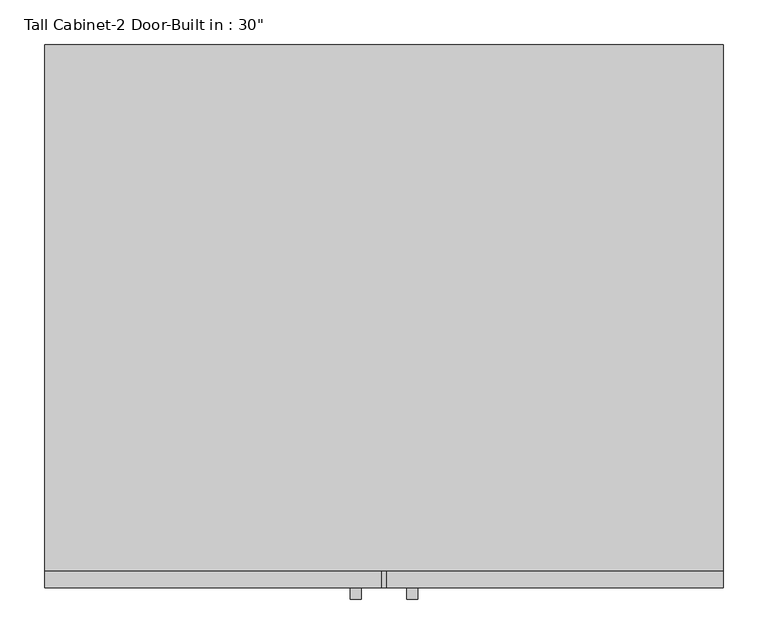
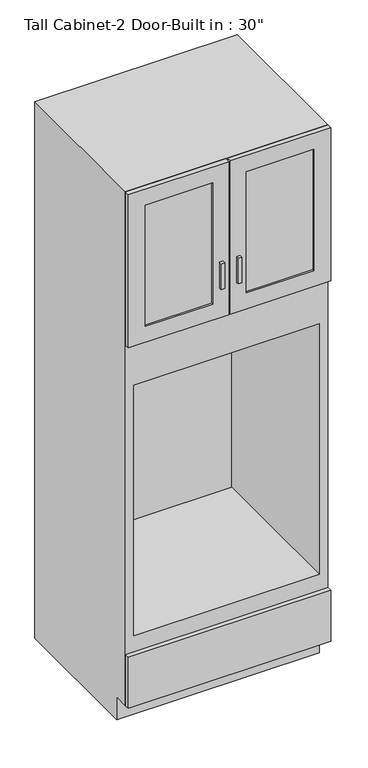
"""IFC4 building model written with IfcOpenShell, lengths in millimetres: furniture geometry."""

from ifc_helpers import new_model, si_unit, frame, origin, place, context, project, spatial, polyline, outline, extrude, faceted_brep, source, transform, mapped, element, save


def furniture_fb6977ac(model_context):
    return source(origin(), model_context, "Body", "SolidModel", [
        faceted_brep([(399.7377049, -590.55, 90.4875), (399.7377049, -590.55, 2135.1875), (-362.2622951, -590.55, 2135.1875), (-362.2622951, -590.55, 90.4875), (-343.2122951, -590.55, 2116.1375), (380.6877049, -590.55, 2116.1375), (380.6877049, -590.55, 1525.5875), (-343.2122951, -590.55, 1525.5875), (367.9877049, -590.55, 357.1875), (-330.5122951, -590.55, 357.1875), (-330.5122951, -590.55, 1354.1375), (367.9877049, -590.55, 1354.1375), (-362.2622951, 0.0, 2135.1875), (399.7377049, 0.0, 2135.1875), (399.7377049, 0.0, 0.0), (-362.2622951, 0.0, 0.0), (399.7377049, -533.4, 90.4875), (399.7377049, -533.4, 0.0), (-362.2622951, -533.4, 0.0), (-362.2622951, -533.4, 90.4875), (380.6877049, -19.05, 2116.1375), (380.6877049, -19.05, 1525.5875), (-343.2122951, -19.05, 1525.5875), (-343.2122951, -19.05, 2116.1375), (367.9877049, -19.05, 357.1875), (-330.5122951, -19.05, 357.1875), (-330.5122951, -19.05, 1354.1375), (367.9877049, -19.05, 1354.1375)], [[[0, 1, 2, 3], [4, 5, 6, 7], [8, 9, 10, 11]], [[12, 13, 14, 15]], [[1, 0, 16, 17, 14, 13]], [[2, 1, 13, 12]], [[3, 2, 12, 15, 18, 19]], [[0, 3, 19, 16]], [[6, 5, 20, 21]], [[4, 7, 22, 23]], [[5, 4, 23, 20]], [[14, 17, 18, 15]], [[18, 17, 16, 19]], [[7, 6, 21, 22]], [[9, 8, 24, 25]], [[10, 9, 25, 26]], [[11, 10, 26, 27]], [[8, 11, 27, 24]], [[21, 20, 23, 22]], [[25, 24, 27, 26]]]),
        extrude(outline(polyline([(399.7377049, -609.6), (-362.2622951, -609.6), (-362.2622951, -590.55), (399.7377049, -590.55), (399.7377049, -609.6)])), frame((0.0, 0.0, 90.4875), z_axis=(0.0, 0.0, 1.0), x_axis=(1.0, 0.0, 0.0)), (0.0, 0.0, 1.0), 203.2),
        extrude(outline(polyline([(2135.1875, 15.5627049), (2135.1875, -362.2622951), (1525.5875, -362.2622951), (1525.5875, 15.5627049), (2135.1875, 15.5627049)]), holes=[polyline([(2071.6875, -44.7622951), (1589.0875, -44.7622951), (1589.0875, -298.7622951), (2071.6875, -298.7622951), (2071.6875, -44.7622951)])]), frame((0.0, -609.6, 0.0), z_axis=(0.0, 1.0, 0.0), x_axis=(0.0, 0.0, 1.0)), (0.0, 0.0, 1.0), 19.05),
        extrude(outline(polyline([(2135.1875, 21.9127049), (1525.5875, 21.9127049), (1525.5875, 399.7377049), (2135.1875, 399.7377049), (2135.1875, 21.9127049)]), holes=[polyline([(2071.6875, 336.2377049), (1589.0875, 336.2377049), (1589.0875, 82.2377049), (2071.6875, 82.2377049), (2071.6875, 336.2377049)])]), frame((0.0, -609.6, 0.0), z_axis=(0.0, 1.0, 0.0), x_axis=(0.0, 0.0, 1.0)), (0.0, 0.0, 1.0), 19.05),
        extrude(outline(polyline([(399.7377049, -609.6), (-362.2622951, -609.6), (-362.2622951, -590.55), (399.7377049, -590.55), (399.7377049, -609.6)])), frame((0.0, 0.0, 90.4875), z_axis=(0.0, 0.0, 1.0), x_axis=(1.0, 0.0, 0.0)), (0.0, 0.0, 1.0), 203.2),
        extrude(outline(polyline([(-6.6622951, -622.3), (-19.1945267, -622.3), (-19.1945267, -609.6), (-6.6622951, -609.6), (-6.6622951, -622.3)])), frame((0.0, 0.0, 1645.6417867), z_axis=(0.0, 0.0, 1.0), x_axis=(1.0, 0.0, 0.0)), (0.0, 0.0, 1.0), 101.6),
        extrude(outline(polyline([(56.6699365, -622.3), (44.1377049, -622.3), (44.1377049, -609.6), (56.6699365, -609.6), (56.6699365, -622.3)])), frame((0.0, 0.0, 1645.6417867), z_axis=(0.0, 0.0, 1.0), x_axis=(1.0, 0.0, 0.0)), (0.0, 0.0, 1.0), 101.6),
        extrude(outline(polyline([(-44.7622951, -603.25), (-298.7622951, -603.25), (-298.7622951, -596.9), (-44.7622951, -596.9), (-44.7622951, -603.25)])), frame((0.0, 0.0, 1589.0875), z_axis=(0.0, 0.0, 1.0), x_axis=(1.0, 0.0, 0.0)), (0.0, 0.0, 1.0), 482.6),
        extrude(outline(polyline([(336.2377049, -603.25), (82.2377049, -603.25), (82.2377049, -596.9), (336.2377049, -596.9), (336.2377049, -603.25)])), frame((0.0, 0.0, 1589.0875), z_axis=(0.0, 0.0, 1.0), x_axis=(1.0, 0.0, 0.0)), (0.0, 0.0, 1.0), 482.6),
    ])


if __name__ == "__main__":
    model = new_model("IFC4")
    model_context = context("Model", 3, world=origin())
    ifc_project = project(units=[si_unit("LENGTHUNIT", "METRE", prefix="MILLI")], contexts=[model_context])
    site = spatial("IfcSite", under=ifc_project)
    building = spatial("IfcBuilding", under=site)
    placement = place(None, origin())
    furniture_shape = furniture_fb6977ac(model_context)
    element("IfcFurniture", 1, ObjectType="Tall Cabinet-2 Door-Built in : 30\"", at=placement, inside=building, context=model_context, shape_type="MappedRepresentation", body=[
        mapped(furniture_shape, transform((0.0, 0.0, 0.0), x_axis=(1.0, 0.0, 0.0), y_axis=(0.0, 1.0, 0.0), z_axis=(0.0, 0.0, 1.0))),
    ])
    save(model, "model.ifc")

# Revit data of these elements
# Type "Tall Cabinet-2 Door-Built in : 30\""
#   Assembly Code = "C1030410"
#   Height = 7' - 0"
#   Depth = 2' - 0"
#   Height-Base of Built-in = 1' - 2"
#   Height-Built-in = 3' - 3 1/4"
#   Height-Upper Cabinet = 2' - 0"
#   Toe Depth = 0' - 3"
#   Toe Height = 0' - 3 1/2"
#   Width = 2' - 6"
#   Cabinet Material = none
#   Door/Drawer Material = none
#   Handle Material = Cabinets - Handles
#   Panel Material = Glass
#   Default Elevation = 0
#   Type Comments = ""
# Element 1 (IfcFurniture, "Tall Cabinet-2 Door-Built in : 30\"")
#   Materials on its faces: "Cabinets", "Cabinets - Handles", "Glass"
# Materials
#   "Cabinets - Handles": class "Metal", colour RGB 57 57 57, transparency 0
#   "Glass": class "Glass", colour RGB 0 128 192, transparency 0.75, Description = "Soda Lime Glass", Cost = 0
#   "Cabinets": colour RGB 249 249 249, transparency 0
